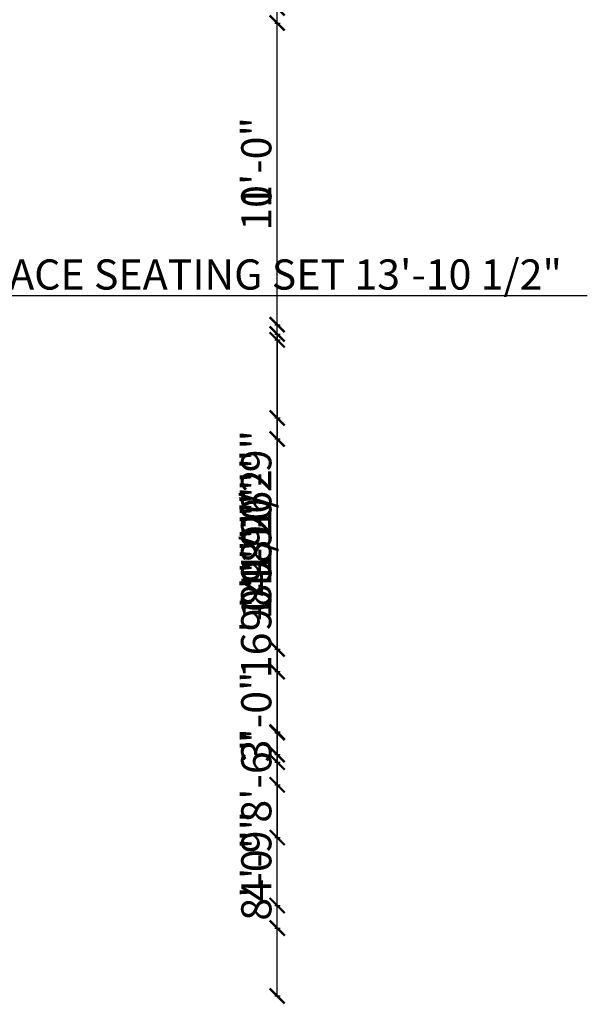
# Model space of a CAD drawing. Units: inches. Extents: x 261 to 2725, y 291 to 1454.
# Tile 33 of 35: x 2500 to 2725, y 409 to 801. Entities that reach past the tile are written whole.
import ezdxf

# ---------------------------------------------------------------- set-up
doc = ezdxf.new("R2010")
doc.units = ezdxf.units.IN
doc.layers.add('A-ANNO-DIMS', color=136, linetype='Continuous', lineweight=18)
doc.styles.get("Standard").update_dxf_attribs({"font": 'arial.ttf'})
doc.dimstyles.new('ISO-25', dxfattribs={"dimtxt": 12, "dimasz": 6, "dimexe": 1.25, "dimexo": 0.625, "dimtad": 1, "dimdec": 0, "dimlunit": 3, "dimtxsty": 'Standard', "dimblk": 'ARCHTICK', "dimcen": 2.5, "dimadec": 0, "dimazin": 0, "dimtfac": 1, "dimtdec": 0, "dimtmove": 0, "dimatfit": 3, "dimfxl": 1, "dimfxlon": 1, "dimarcsym": 0})

# ---------------------------------------------------------------- blocks, each defined once
blk = doc.blocks.new('_ArchTick')
at = {"color": 0, "linetype": 'ByBlock', "const_width": 0.15}
blk.add_lwpolyline([(-0.5, -0.5), (0.5, 0.5)], dxfattribs=at)
blk = doc.blocks.new('*D71')
at = {"layer": 'A-ANNO-DIMS', "color": 0, "lineweight": -2, "ltscale": 0.07, "transparency": 16777216}
for p, q in [((2272.38, 690.06), (2272.38, 692.31)), ((2272.38, 691.06), (2439.01, 691.06)), ((2439.01, 690.06), (2439.01, 692.31)), ((2439.01, 691.06), (2725.34, 691.06))]:
    blk.add_line(p, q, dxfattribs=at)
at = {"layer": 'Defpoints', "color": 0, "ltscale": 0.07, "transparency": 16777216}
for p in [(2439.01, 691.06), (2272.38, 666.07), (2439.01, 666.07)]:
    blk.add_point(p, dxfattribs=at)
at = {"layer": 'A-ANNO-DIMS', "color": 0, "lineweight": -2, "ltscale": 0.07, "transparency": 16777216, "xscale": 6, "yscale": 6, "zscale": 6, "rotation": 180}
blk.add_blockref('_ArchTick', (2272.38, 691.06), dxfattribs=at)
at = {"layer": 'A-ANNO-DIMS', "color": 0, "lineweight": -2, "ltscale": 0.07, "transparency": 16777216, "xscale": 6, "yscale": 6, "zscale": 6}
blk.add_blockref('_ArchTick', (2439.01, 691.06), dxfattribs=at)
at = {"layer": 'A-ANNO-DIMS', "color": 0, "ltscale": 0.07, "transparency": 16777216, "insert": (2585.18, 697.9), "char_height": 12, "attachment_point": 5}
blk.add_mtext('TERRACE SEATING SET 13\'-10 1/2"', dxfattribs=at)
blk = doc.blocks.new('*D82')
at = {"layer": 'A-ANNO-DIMS', "color": 0, "lineweight": -2, "ltscale": 0.07, "transparency": 16777216}
for p, q in [((2600.96, 679.47), (2603.21, 679.47)), ((2601.96, 517.47), (2601.96, 679.47)), ((2600.96, 517.47), (2603.21, 517.47))]:
    blk.add_line(p, q, dxfattribs=at)
at = {"layer": 'Defpoints', "color": 0, "ltscale": 0.07, "transparency": 16777216}
for p in [(946.45, 679.47), (2601.96, 679.47), (946.45, 517.47)]:
    blk.add_point(p, dxfattribs=at)
at = {"layer": 'A-ANNO-DIMS', "color": 0, "lineweight": -2, "ltscale": 0.07, "transparency": 16777216, "xscale": 6, "yscale": 6, "zscale": 6}
for p, rotation in [((2601.96, 679.47), 90), ((2601.96, 517.47), 270)]:
    blk.add_blockref('_ArchTick', p, dxfattribs=dict(at, rotation=rotation))
at = {"layer": 'A-ANNO-DIMS', "color": 0, "ltscale": 0.07, "transparency": 16777216, "insert": (2595.2, 598.47), "char_height": 12, "attachment_point": 5, "rotation": 90}
blk.add_mtext('13\'-6"', dxfattribs=at)
blk = doc.blocks.new('*D83')
at = {"layer": 'A-ANNO-DIMS', "color": 0, "lineweight": -2, "ltscale": 0.07, "transparency": 16777216}
for p, q in [((2600.96, 799.47), (2603.21, 799.47)), ((2601.96, 679.47), (2601.96, 799.47)), ((2600.96, 679.47), (2603.21, 679.47))]:
    blk.add_line(p, q, dxfattribs=at)
at = {"layer": 'Defpoints', "color": 0, "ltscale": 0.07, "transparency": 16777216}
for p in [(946.45, 799.47), (2601.96, 799.47), (946.45, 679.47)]:
    blk.add_point(p, dxfattribs=at)
at = {"layer": 'A-ANNO-DIMS', "color": 0, "lineweight": -2, "ltscale": 0.07, "transparency": 16777216, "xscale": 6, "yscale": 6, "zscale": 6}
for p, rotation in [((2601.96, 799.47), 90), ((2601.96, 679.47), 270)]:
    blk.add_blockref('_ArchTick', p, dxfattribs=dict(at, rotation=rotation))
at = {"layer": 'A-ANNO-DIMS', "color": 0, "ltscale": 0.07, "transparency": 16777216, "insert": (2595.21, 739.47), "char_height": 12, "attachment_point": 5, "rotation": 90}
blk.add_mtext('10\'-0"', dxfattribs=at)
blk = doc.blocks.new('*D84')
at = {"layer": 'A-ANNO-DIMS', "color": 0, "lineweight": -2, "ltscale": 0.07, "transparency": 16777216}
for p, q in [((2600.96, 1024.47), (2603.21, 1024.47)), ((2601.96, 799.47), (2601.96, 1024.47)), ((2600.96, 799.47), (2603.21, 799.47))]:
    blk.add_line(p, q, dxfattribs=at)
at = {"layer": 'Defpoints', "color": 0, "ltscale": 0.07, "transparency": 16777216}
for p in [(946.45, 1024.47), (2601.96, 1024.47), (946.45, 799.47)]:
    blk.add_point(p, dxfattribs=at)
at = {"layer": 'A-ANNO-DIMS', "color": 0, "lineweight": -2, "ltscale": 0.07, "transparency": 16777216, "xscale": 6, "yscale": 6, "zscale": 6}
for p, rotation in [((2601.96, 1024.47), 90), ((2601.96, 799.47), 270)]:
    blk.add_blockref('_ArchTick', p, dxfattribs=dict(at, rotation=rotation))
at = {"layer": 'A-ANNO-DIMS', "color": 0, "ltscale": 0.07, "transparency": 16777216, "insert": (2595.21, 911.97), "char_height": 12, "attachment_point": 5, "rotation": 90}
blk.add_mtext('18\'-9"', dxfattribs=at)
blk = doc.blocks.new('*D89')
at = {"layer": 'A-ANNO-DIMS', "color": 0, "lineweight": -2, "ltscale": 0.07, "transparency": 16777216}
for p, q in [((2600.96, 508.47), (2603.21, 508.47)), ((2601.96, 412.47), (2601.96, 508.47)), ((2600.96, 412.47), (2603.21, 412.47))]:
    blk.add_line(p, q, dxfattribs=at)
at = {"layer": 'Defpoints', "color": 0, "ltscale": 0.07, "transparency": 16777216}
for p in [(955.45, 508.47), (2601.96, 508.47), (994.45, 412.47)]:
    blk.add_point(p, dxfattribs=at)
at = {"layer": 'A-ANNO-DIMS', "color": 0, "lineweight": -2, "ltscale": 0.07, "transparency": 16777216, "xscale": 6, "yscale": 6, "zscale": 6}
for p, rotation in [((2601.96, 508.47), 90), ((2601.96, 412.47), 270)]:
    blk.add_blockref('_ArchTick', p, dxfattribs=dict(at, rotation=rotation))
at = {"layer": 'A-ANNO-DIMS', "color": 0, "ltscale": 0.07, "transparency": 16777216, "insert": (2595.21, 460.47), "char_height": 12, "attachment_point": 5, "rotation": 90}
blk.add_mtext('8\'-0"', dxfattribs=at)
blk = doc.blocks.new('*D111')
at = {"layer": 'A-ANNO-DIMS', "color": 0, "lineweight": -2, "ltscale": 0.07, "transparency": 16777216}
for p, q in [((2600.96, 550.47), (2603.21, 550.47)), ((2601.96, 448.47), (2601.96, 550.47)), ((2600.96, 448.47), (2603.21, 448.47))]:
    blk.add_line(p, q, dxfattribs=at)
at = {"layer": 'Defpoints', "color": 0, "ltscale": 0.07, "transparency": 16777216}
for p in [(1720.08, 550.47), (2601.96, 550.47), (1720.08, 448.47)]:
    blk.add_point(p, dxfattribs=at)
at = {"layer": 'A-ANNO-DIMS', "color": 0, "lineweight": -2, "ltscale": 0.07, "transparency": 16777216, "xscale": 6, "yscale": 6, "zscale": 6}
for p, rotation in [((2601.96, 550.47), 90), ((2601.96, 448.47), 270)]:
    blk.add_blockref('_ArchTick', p, dxfattribs=dict(at, rotation=rotation))
at = {"layer": 'A-ANNO-DIMS', "color": 0, "ltscale": 0.07, "transparency": 16777216, "insert": (2595.21, 499.47), "char_height": 12, "attachment_point": 5, "rotation": 90}
blk.add_mtext('8\'-6"', dxfattribs=at)
blk = doc.blocks.new('*D112')
at = {"layer": 'A-ANNO-DIMS', "color": 0, "lineweight": -2, "ltscale": 0.07, "transparency": 16777216}
for p, q in [((2600.96, 679.47), (2603.21, 679.47)), ((2601.96, 550.47), (2601.96, 679.47)), ((2600.96, 550.47), (2603.21, 550.47))]:
    blk.add_line(p, q, dxfattribs=at)
at = {"layer": 'Defpoints', "color": 0, "ltscale": 0.07, "transparency": 16777216}
for p in [(1720.08, 679.47), (2601.96, 679.47), (1720.08, 550.47)]:
    blk.add_point(p, dxfattribs=at)
at = {"layer": 'A-ANNO-DIMS', "color": 0, "lineweight": -2, "ltscale": 0.07, "transparency": 16777216, "xscale": 6, "yscale": 6, "zscale": 6}
for p, rotation in [((2601.96, 679.47), 90), ((2601.96, 550.47), 270)]:
    blk.add_blockref('_ArchTick', p, dxfattribs=dict(at, rotation=rotation))
at = {"layer": 'A-ANNO-DIMS', "color": 0, "ltscale": 0.07, "transparency": 16777216, "insert": (2595.21, 614.97), "char_height": 12, "attachment_point": 5, "rotation": 90}
blk.add_mtext('10\'-9"', dxfattribs=at)
blk = doc.blocks.new('*D113')
at = {"layer": 'A-ANNO-DIMS', "color": 0, "lineweight": -2, "ltscale": 0.07, "transparency": 16777216}
for p, q in [((2600.96, 799.47), (2603.21, 799.47)), ((2601.96, 679.47), (2601.96, 799.47)), ((2600.96, 679.47), (2603.21, 679.47))]:
    blk.add_line(p, q, dxfattribs=at)
at = {"layer": 'Defpoints', "color": 0, "ltscale": 0.07, "transparency": 16777216}
for p in [(1720.08, 799.47), (2601.96, 799.47), (1720.08, 679.47)]:
    blk.add_point(p, dxfattribs=at)
at = {"layer": 'A-ANNO-DIMS', "color": 0, "lineweight": -2, "ltscale": 0.07, "transparency": 16777216, "xscale": 6, "yscale": 6, "zscale": 6}
for p, rotation in [((2601.96, 799.47), 90), ((2601.96, 679.47), 270)]:
    blk.add_blockref('_ArchTick', p, dxfattribs=dict(at, rotation=rotation))
at = {"layer": 'A-ANNO-DIMS', "color": 0, "ltscale": 0.07, "transparency": 16777216, "insert": (2595.21, 739.47), "char_height": 12, "attachment_point": 5, "rotation": 90}
blk.add_mtext('10\'-0"', dxfattribs=at)
blk = doc.blocks.new('*D114')
at = {"layer": 'A-ANNO-DIMS', "color": 0, "lineweight": -2, "ltscale": 0.07, "transparency": 16777216}
for p, q in [((2600.96, 964.47), (2603.21, 964.47)), ((2601.96, 799.47), (2601.96, 964.47)), ((2600.96, 799.47), (2603.21, 799.47))]:
    blk.add_line(p, q, dxfattribs=at)
at = {"layer": 'Defpoints', "color": 0, "ltscale": 0.07, "transparency": 16777216}
for p in [(1720.08, 964.47), (2601.96, 964.47), (1720.08, 799.47)]:
    blk.add_point(p, dxfattribs=at)
at = {"layer": 'A-ANNO-DIMS', "color": 0, "lineweight": -2, "ltscale": 0.07, "transparency": 16777216, "xscale": 6, "yscale": 6, "zscale": 6}
for p, rotation in [((2601.96, 964.47), 90), ((2601.96, 799.47), 270)]:
    blk.add_blockref('_ArchTick', p, dxfattribs=dict(at, rotation=rotation))
at = {"layer": 'A-ANNO-DIMS', "color": 0, "ltscale": 0.07, "transparency": 16777216, "insert": (2595.2, 881.97), "char_height": 12, "attachment_point": 5, "rotation": 90}
blk.add_mtext('13\'-9"', dxfattribs=at)
blk = doc.blocks.new('*D125')
at = {"layer": 'A-ANNO-DIMS', "color": 0, "lineweight": -2, "ltscale": 0.07, "transparency": 16777216}
for p, q in [((2600.96, 496.47), (2603.21, 496.47)), ((2601.96, 439.47), (2601.96, 496.47)), ((2600.96, 439.47), (2603.21, 439.47))]:
    blk.add_line(p, q, dxfattribs=at)
at = {"layer": 'Defpoints', "color": 0, "ltscale": 0.07, "transparency": 16777216}
for p in [(2214.67, 496.47), (2601.96, 496.47), (2214.67, 439.47)]:
    blk.add_point(p, dxfattribs=at)
at = {"layer": 'A-ANNO-DIMS', "color": 0, "lineweight": -2, "ltscale": 0.07, "transparency": 16777216, "xscale": 6, "yscale": 6, "zscale": 6}
for p, rotation in [((2601.96, 496.47), 90), ((2601.96, 439.47), 270)]:
    blk.add_blockref('_ArchTick', p, dxfattribs=dict(at, rotation=rotation))
at = {"layer": 'A-ANNO-DIMS', "color": 0, "ltscale": 0.07, "transparency": 16777216, "insert": (2595.21, 467.97), "char_height": 12, "attachment_point": 5, "rotation": 90}
blk.add_mtext('4\'-9"', dxfattribs=at)
blk = doc.blocks.new('*D126')
at = {"layer": 'A-ANNO-DIMS', "color": 0, "lineweight": -2, "ltscale": 0.07, "transparency": 16777216}
for p, q in [((2600.96, 673.47), (2603.21, 673.47)), ((2601.96, 496.47), (2601.96, 673.47)), ((2600.96, 496.47), (2603.21, 496.47))]:
    blk.add_line(p, q, dxfattribs=at)
at = {"layer": 'Defpoints', "color": 0, "ltscale": 0.07, "transparency": 16777216}
for p in [(2484.71, 673.47), (2601.96, 673.47), (2493.71, 496.47)]:
    blk.add_point(p, dxfattribs=at)
at = {"layer": 'A-ANNO-DIMS', "color": 0, "lineweight": -2, "ltscale": 0.07, "transparency": 16777216, "xscale": 6, "yscale": 6, "zscale": 6}
for p, rotation in [((2601.96, 673.47), 90), ((2601.96, 496.47), 270)]:
    blk.add_blockref('_ArchTick', p, dxfattribs=dict(at, rotation=rotation))
at = {"layer": 'A-ANNO-DIMS', "color": 0, "ltscale": 0.07, "transparency": 16777216, "insert": (2595.21, 584.97), "char_height": 12, "attachment_point": 5, "rotation": 90}
blk.add_mtext('14\'-9"', dxfattribs=at)
blk = doc.blocks.new('*D127')
at = {"layer": 'A-ANNO-DIMS', "color": 0, "lineweight": -2, "ltscale": 0.07, "transparency": 16777216}
for p, q in [((2600.96, 805.47), (2603.21, 805.47)), ((2601.96, 673.47), (2601.96, 805.47)), ((2600.96, 673.47), (2603.21, 673.47))]:
    blk.add_line(p, q, dxfattribs=at)
at = {"layer": 'Defpoints', "color": 0, "ltscale": 0.07, "transparency": 16777216}
for p in [(2484.71, 805.47), (2601.96, 805.47), (2484.71, 673.47)]:
    blk.add_point(p, dxfattribs=at)
at = {"layer": 'A-ANNO-DIMS', "color": 0, "lineweight": -2, "ltscale": 0.07, "transparency": 16777216, "xscale": 6, "yscale": 6, "zscale": 6}
for p, rotation in [((2601.96, 805.47), 90), ((2601.96, 673.47), 270)]:
    blk.add_blockref('_ArchTick', p, dxfattribs=dict(at, rotation=rotation))
at = {"layer": 'A-ANNO-DIMS', "color": 0, "ltscale": 0.07, "transparency": 16777216, "insert": (2595.21, 739.47), "char_height": 12, "attachment_point": 5, "rotation": 90}
blk.add_mtext('11\'-0"', dxfattribs=at)
blk = doc.blocks.new('*D130')
at = {"layer": 'A-ANNO-DIMS', "color": 0, "lineweight": -2, "ltscale": 0.07, "transparency": 16777216}
for p, q in [((2600.96, 541.47), (2603.21, 541.47)), ((2601.96, 505.47), (2601.96, 541.47)), ((2600.96, 505.47), (2603.21, 505.47))]:
    blk.add_line(p, q, dxfattribs=at)
at = {"layer": 'Defpoints', "color": 0, "ltscale": 0.07, "transparency": 16777216}
for p in [(2448.71, 541.47), (2601.96, 541.47), (2484.71, 505.47)]:
    blk.add_point(p, dxfattribs=at)
at = {"layer": 'A-ANNO-DIMS', "color": 0, "lineweight": -2, "ltscale": 0.07, "transparency": 16777216, "xscale": 6, "yscale": 6, "zscale": 6}
for p, rotation in [((2601.96, 541.47), 90), ((2601.96, 505.47), 270)]:
    blk.add_blockref('_ArchTick', p, dxfattribs=dict(at, rotation=rotation))
at = {"layer": 'A-ANNO-DIMS', "color": 0, "ltscale": 0.07, "transparency": 16777216, "insert": (2595.2, 523.47), "char_height": 12, "attachment_point": 5, "rotation": 90}
blk.add_mtext('3\'-0"', dxfattribs=at)
blk = doc.blocks.new('*D136')
at = {"layer": 'A-ANNO-DIMS', "color": 0, "lineweight": -2, "ltscale": 0.07, "transparency": 16777216}
for p, q in [((2600.96, 675.78), (2603.21, 675.78)), ((2601.96, 675.78), (2601.96, 475.47)), ((2600.96, 475.47), (2603.21, 475.47))]:
    blk.add_line(p, q, dxfattribs=at)
at = {"layer": 'Defpoints', "color": 0, "ltscale": 0.07, "transparency": 16777216}
for p in [(2208.67, 675.78), (2208.67, 475.47), (2601.96, 475.47)]:
    blk.add_point(p, dxfattribs=at)
at = {"layer": 'A-ANNO-DIMS', "color": 0, "lineweight": -2, "ltscale": 0.07, "transparency": 16777216, "xscale": 6, "yscale": 6, "zscale": 6}
for p, rotation in [((2601.96, 675.78), 90), ((2601.96, 475.47), 270)]:
    blk.add_blockref('_ArchTick', p, dxfattribs=dict(at, rotation=rotation))
at = {"layer": 'A-ANNO-DIMS', "color": 0, "ltscale": 0.07, "transparency": 16777216, "insert": (2595.13, 575.62), "char_height": 12, "attachment_point": 5, "rotation": 90}
blk.add_mtext('16\'-8 1/2"', dxfattribs=at)
blk = doc.blocks.new('*D137')
at = {"layer": 'A-ANNO-DIMS', "color": 0, "lineweight": -2, "ltscale": 0.07, "transparency": 16777216}
for p, q in [((2600.96, 642.39), (2603.21, 642.39)), ((2601.96, 642.39), (2601.96, 634.05)), ((2600.96, 634.05), (2603.21, 634.05)), ((2601.96, 634.05), (2601.96, 566.94))]:
    blk.add_line(p, q, dxfattribs=at)
at = {"layer": 'Defpoints', "color": 0, "ltscale": 0.07, "transparency": 16777216}
for p in [(2221.19, 642.39), (2221.19, 634.05), (2601.96, 634.05)]:
    blk.add_point(p, dxfattribs=at)
at = {"layer": 'A-ANNO-DIMS', "color": 0, "lineweight": -2, "ltscale": 0.07, "transparency": 16777216, "xscale": 6, "yscale": 6, "zscale": 6}
for p, rotation in [((2601.96, 642.39), 90), ((2601.96, 634.05), 270)]:
    blk.add_blockref('_ArchTick', p, dxfattribs=dict(at, rotation=rotation))
at = {"layer": 'A-ANNO-DIMS', "color": 0, "ltscale": 0.07, "transparency": 16777216, "insert": (2595.13, 597.49), "char_height": 12, "attachment_point": 5, "rotation": 90}
blk.add_mtext('0\'-8 1/2"', dxfattribs=at)
blk = doc.blocks.new('*D138')
at = {"layer": 'A-ANNO-DIMS', "color": 0, "lineweight": -2, "ltscale": 0.07, "transparency": 16777216}
for p, q in [((2600.96, 634.05), (2603.21, 634.05)), ((2601.96, 634.05), (2601.96, 517.2)), ((2600.96, 517.2), (2603.21, 517.2))]:
    blk.add_line(p, q, dxfattribs=at)
at = {"layer": 'Defpoints', "color": 0, "ltscale": 0.07, "transparency": 16777216}
for p in [(2221.19, 634.05), (2221.19, 517.2), (2601.96, 517.2)]:
    blk.add_point(p, dxfattribs=at)
at = {"layer": 'A-ANNO-DIMS', "color": 0, "lineweight": -2, "ltscale": 0.07, "transparency": 16777216, "xscale": 6, "yscale": 6, "zscale": 6}
for p, rotation in [((2601.96, 634.05), 90), ((2601.96, 517.2), 270)]:
    blk.add_blockref('_ArchTick', p, dxfattribs=dict(at, rotation=rotation))
at = {"layer": 'A-ANNO-DIMS', "color": 0, "ltscale": 0.07, "transparency": 16777216, "insert": (2595.21, 575.62), "char_height": 12, "attachment_point": 5, "rotation": 90}
blk.add_mtext('9\'-9"', dxfattribs=at)

msp = doc.modelspace()

# ---------------------------------------------------------------- dimensions: what is measured, and where the dimension line sits
at = {"layer": 'A-ANNO-DIMS', "ltscale": 0.07}
for base, p1, p2, picture, middle in [((2601.96, 1024.47), (946.45, 799.47), (946.45, 1024.47), '*D84', (2595.21, 911.97)), ((2601.96, 964.47), (1720.08, 799.47), (1720.08, 964.47), '*D114', (2595.2, 881.97)), ((2601.96, 805.47), (2484.71, 673.47), (2484.71, 805.47), '*D127', (2595.21, 739.47)), ((2601.96, 799.47), (946.45, 679.47), (946.45, 799.47), '*D83', (2595.21, 739.47)), ((2601.96, 799.47), (1720.08, 679.47), (1720.08, 799.47), '*D113', (2595.21, 739.47)), ((2601.96, 679.47), (946.45, 517.47), (946.45, 679.47), '*D82', (2595.2, 598.47)), ((2601.96, 679.47), (1720.08, 550.47), (1720.08, 679.47), '*D112', (2595.21, 614.97)), ((2601.96, 475.47), (2208.67, 675.78), (2208.67, 475.47), '*D136', (2595.13, 575.62)), ((2601.96, 673.47), (2493.71, 496.47), (2484.71, 673.47), '*D126', (2595.21, 584.97)), ((2601.96, 634.05), (2221.19, 642.39), (2221.19, 634.05), '*D137', (2595.13, 597.49)), ((2601.9578, 517.1998), (2221.1928, 634.0483), (2221.1928, 517.1998), '*D138', (2595.2059, 575.6241)), ((2601.96, 550.47), (1720.08, 448.47), (1720.08, 550.47), '*D111', (2595.21, 499.47)), ((2601.96, 541.47), (2484.71, 505.47), (2448.71, 541.47), '*D130', (2595.2, 523.47)), ((2601.96, 508.47), (994.45, 412.47), (955.45, 508.47), '*D89', (2595.21, 460.47)), ((2601.96, 496.47), (2214.67, 439.47), (2214.67, 496.47), '*D125', (2595.21, 467.97))]:
    dim = msp.add_linear_dim(base=base, p1=p1, p2=p2, angle=90, dimstyle='ISO-25', override={"dimdec": 1, "dimlfac": 1, "dimrnd": 0, "dimzin": 1, "dimdsep": 46, "dimlunit": 4, "dimfrac": 2}, dxfattribs=at)
    dim.commit()
    dim.dimension.update_dxf_attribs({"geometry": picture, "text_midpoint": middle})
dim = msp.add_linear_dim(base=(2439.01, 691.06), p1=(2272.38, 666.07), p2=(2439.01, 666.07), text='TERRACE SEATING SET <>', dimstyle='ISO-25', override={"dimdec": 1, "dimrnd": 0, "dimzin": 1, "dimlunit": 4, "dimfrac": 2}, dxfattribs=at)
dim.commit()
dim.dimension.update_dxf_attribs({"geometry": '*D71', "text_midpoint": (2585.18, 697.9)})

doc.saveas('drawing.dxf')
